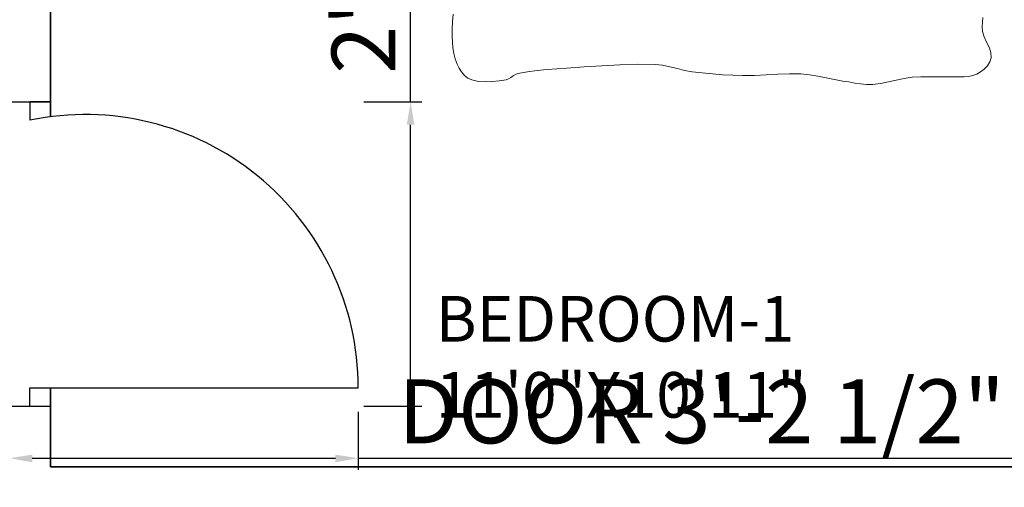
# Model space of a CAD drawing. Units: inches. Extents: x 1484 to 2008, y 1843 to 2590.
# Tile 11 of 21: x 1756 to 1864, y 2075 to 2126. Entities that reach past the tile are written whole.
import ezdxf

# ---------------------------------------------------------------- set-up
doc = ezdxf.new("R2010")
doc.units = ezdxf.units.IN
for name, color, linetype, lineweight in [('A-ANNO-DIMS', 2, 'Continuous', 18), ('A-AREA-IDEN', 7, 'Continuous', 18), ('A-DOOR', 4, 'Continuous', 25), ('A-FURN', 8, 'Continuous', 18), ('A-WALL', 7, 'Continuous', 35)]:
    doc.layers.add(name, color=color, linetype=linetype, lineweight=lineweight)
doc.styles.get("Standard").update_dxf_attribs({"font": 'arial.ttf'})
doc.dimstyles.new('ISO-25', dxfattribs={"dimtxt": 7, "dimasz": 2.5, "dimexe": 1.25, "dimexo": 0.625, "dimtad": 1, "dimdec": 0, "dimlunit": 3, "dimtxsty": 'Standard', "dimcen": 2.5, "dimadec": 0, "dimazin": 0, "dimtfac": 1, "dimtdec": 0, "dimtmove": 0, "dimatfit": 3, "dimfxl": 1, "dimarcsym": 0})

# ---------------------------------------------------------------- blocks, each defined once
blk = doc.blocks.new('BED-DOUBLE')
for p, q in [((0.44, 7.72), (0.38, 6.9)), ((0.38, 6.9), (0.33, 6.08)), ((58.47, 6.32), (58.48, 6.84)), ((58.48, 6.84), (58.53, 7.36)), ((0.33, 6.08), (0.34, 5.26)), ((58.51, 5.8), (58.47, 6.32)), ((58.67, 5.21), (58.51, 5.8)), ((0.34, 5.26), (0.37, 4.64)), ((0.37, 4.64), (0.43, 4.02)), ((58.94, 4.64), (58.67, 5.21)), ((59.21, 4.08), (58.94, 4.64)), ((0.43, 4.02), (0.52, 3.41)), ((0.52, 3.41), (0.66, 2.81)), ((59.41, 3.51), (59.21, 4.08)), ((59.44, 2.92), (59.41, 3.51)), ((0.66, 2.81), (0.87, 2.24)), ((0.87, 2.24), (1.09, 1.8)), ((16.76, 2.06), (18.71, 2.17)), ((18.71, 2.17), (20.65, 2.22)), ((20.65, 2.22), (22.59, 2.2)), ((22.59, 2.2), (23.41, 2.12)), ((59.04, 2.06), (59.3, 2.47)), ((59.3, 2.47), (59.44, 2.92)), ((1.09, 1.8), (1.37, 1.38)), ((1.37, 1.38), (1.69, 1)), ((7.03, 0.95), (7.28, 1.11)), ((7.28, 1.11), (7.55, 1.21)), ((7.55, 1.21), (8.61, 1.39)), ((8.61, 1.39), (9.67, 1.53)), ((9.67, 1.53), (10.74, 1.64)), ((10.74, 1.64), (11.81, 1.73)), ((11.81, 1.73), (12.88, 1.8)), ((12.88, 1.8), (14.82, 1.94)), ((14.82, 1.94), (16.76, 2.06)), ((23.41, 2.12), (24.22, 1.95)), ((24.22, 1.95), (25.03, 1.75)), ((25.03, 1.75), (25.83, 1.54)), ((25.83, 1.54), (26.65, 1.4)), ((26.65, 1.4), (27.76, 1.27)), ((27.76, 1.27), (28.88, 1.16)), ((28.88, 1.16), (29.99, 1.07)), ((34.77, 1.05), (36.04, 1.13)), ((36.04, 1.13), (37.32, 1.18)), ((37.32, 1.18), (38.59, 1.16)), ((38.59, 1.16), (39.51, 1.07)), ((57.43, 0.97), (57.87, 1.14)), ((57.87, 1.14), (58.29, 1.39)), ((58.29, 1.39), (58.69, 1.7)), ((58.69, 1.7), (59.04, 2.06)), ((1.69, 1), (2.07, 0.7)), ((2.07, 0.7), (2.5, 0.5)), ((2.5, 0.5), (3.23, 0.34)), ((3.23, 0.34), (3.98, 0.29)), ((3.98, 0.29), (4.74, 0.33)), ((4.74, 0.33), (5.5, 0.41)), ((5.5, 0.41), (6.25, 0.52)), ((6.25, 0.52), (6.53, 0.61)), ((6.53, 0.61), (6.78, 0.77)), ((6.78, 0.77), (7.03, 0.95)), ((29.99, 1.07), (31.11, 1.01)), ((31.11, 1.01), (32.23, 0.97)), ((32.23, 0.97), (33.5, 0.99)), ((33.5, 0.99), (34.77, 1.05)), ((39.51, 1.07), (40.43, 0.92)), ((40.43, 0.92), (41.35, 0.73)), ((41.35, 0.73), (42.27, 0.54)), ((42.27, 0.54), (43.19, 0.38)), ((43.19, 0.38), (43.83, 0.28)), ((43.83, 0.28), (44.48, 0.16)), ((44.48, 0.16), (45.13, 0.06)), ((45.13, 0.06), (45.77, 0)), ((45.77, 0), (46.42, 0)), ((46.42, 0), (47.3, 0.1)), ((47.3, 0.1), (48.17, 0.28)), ((48.17, 0.28), (49.04, 0.48)), ((49.04, 0.48), (49.91, 0.67)), ((49.91, 0.67), (50.79, 0.8)), ((50.79, 0.8), (51.74, 0.85)), ((51.74, 0.85), (52.68, 0.86)), ((52.68, 0.86), (53.63, 0.84)), ((53.63, 0.84), (54.58, 0.83)), ((54.58, 0.83), (55.53, 0.85)), ((55.53, 0.85), (56.01, 0.86)), ((56.01, 0.86), (56.49, 0.86)), ((56.49, 0.86), (56.97, 0.89)), ((56.97, 0.89), (57.43, 0.97))]:
    blk.add_line(p, q)
blk = doc.blocks.new('DOOR-SWING-36IN')
for p, q in [((-2.25, 31.33), (2.25, 31.33)), ((0, 31.33), (0, 29.33)), ((0, -2), (0, 0)), ((0, 0), (36, 0)), ((-2.25, -2), (2.25, -2))]:
    blk.add_line(p, q)
blk.add_arc((6.05, 0), 29.95, 0, 101.6643)
blk = doc.blocks.new('*D11')
at = {"layer": 'A-ANNO-DIMS', "color": 0, "lineweight": -2, "transparency": 16777216}
for p, q in [((1754.42, 2083.34), (1754.42, 2076.98)), ((1792.67, 2083.34), (1792.67, 2076.98)), ((1756.92, 2078.23), (1790.17, 2078.23)), ((1792.67, 2078.23), (1887.1, 2078.23))]:
    blk.add_line(p, q, dxfattribs=at)
at = {"layer": 'A-ANNO-DIMS', "color": 0, "transparency": 16777216}
for points in [[(1756.92, 2078.64), (1756.92, 2077.81), (1754.42, 2078.23)], [(1790.17, 2078.64), (1790.17, 2077.81), (1792.67, 2078.23)]]:
    blk.add_solid(points, dxfattribs=at)
at = {"layer": 'Defpoints', "color": 0, "transparency": 16777216}
for p in [(1754.42, 2083.96), (1792.67, 2083.96), (1792.67, 2078.23)]:
    blk.add_point(p, dxfattribs=at)
at = {"layer": 'A-ANNO-DIMS', "color": 0, "transparency": 16777216, "insert": (1841.14, 2082.47), "char_height": 7, "attachment_point": 5}
blk.add_mtext('DOOR 3\'-2 1/2" TYP.', dxfattribs=at)
blk = doc.blocks.new('*D12')
at = {"layer": 'A-ANNO-DIMS', "color": 0, "lineweight": -2, "transparency": 16777216}
for p, q in [((1798.41, 2117.29), (1798.41, 2180.14)), ((1793.29, 2117.29), (1799.66, 2117.29)), ((1798.41, 2086.46), (1798.41, 2114.79)), ((1793.29, 2083.96), (1799.66, 2083.96))]:
    blk.add_line(p, q, dxfattribs=at)
at = {"layer": 'A-ANNO-DIMS', "color": 0, "transparency": 16777216}
for points in [[(1797.99, 2114.79), (1798.82, 2114.79), (1798.41, 2117.29)], [(1797.99, 2086.46), (1798.82, 2086.46), (1798.41, 2083.96)]]:
    blk.add_solid(points, dxfattribs=at)
at = {"layer": 'Defpoints', "color": 0, "transparency": 16777216}
for p in [(1792.67, 2117.29), (1798.41, 2117.29), (1792.67, 2083.96)]:
    blk.add_point(p, dxfattribs=at)
at = {"layer": 'A-ANNO-DIMS', "color": 0, "transparency": 16777216, "insert": (1794.16, 2149.96), "char_height": 7, "attachment_point": 5, "rotation": 90}
blk.add_mtext('2\'-9 1/2" TYP.', dxfattribs=at)

msp = doc.modelspace()

# ---------------------------------------------------------------- linework, layer by layer
at = {"layer": 'A-DOOR'}
msp.add_line((1758.92, 2117.29), (1756.67, 2117.29), dxfattribs=at)
at = {"layer": 'A-WALL'}
for p, q in [((1758.92, 2208.3), (1758.92, 2115.67)), ((1758.92, 2085.96), (1758.92, 2077.3)), ((1758.92, 2077.3), (1890.92, 2077.3))]:
    msp.add_line(p, q, dxfattribs=at)

# ---------------------------------------------------------------- block references
at = {"layer": 'A-DOOR'}
msp.add_blockref('DOOR-SWING-36IN', (1756.67, 2085.96), dxfattribs=at)
at = {"layer": 'A-FURN'}
msp.add_blockref('BED-DOUBLE', (1802.63, 2119.2), dxfattribs=at)

# ---------------------------------------------------------------- texts
at = {"layer": 'A-AREA-IDEN', "insert": (1801.17, 2096.02), "char_height": 5, "attachment_point": 1}
msp.add_mtext_dynamic_manual_height_columns('BEDROOM-1\\P11\'0"X10\'11"', width=115.7673, gutter_width=12.5, heights=[0], dxfattribs=at)

# ---------------------------------------------------------------- dimensions: what is measured, and where the dimension line sits
at = {"layer": 'A-ANNO-DIMS'}
dim = msp.add_linear_dim(base=(1798.41, 2117.29), p1=(1792.67, 2083.96), p2=(1792.67, 2117.29), angle=90, text='<> TYP.', dimstyle='ISO-25', override={"dimdec": 1, "dimlfac": 1, "dimrnd": 0, "dimzin": 1, "dimdsep": 46, "dimlunit": 4, "dimfrac": 2}, dxfattribs=at)
dim.commit()
dim.dimension.update_dxf_attribs({"geometry": '*D12', "text_midpoint": (1794.16, 2149.96)})
dim = msp.add_linear_dim(base=(1792.66964371, 2078.22557639), p1=(1754.41964371, 2083.96307639), p2=(1792.66964371, 2083.96307639), text='DOOR <> TYP.', dimstyle='ISO-25', override={"dimdec": 1, "dimlfac": 1, "dimrnd": 0, "dimzin": 1, "dimdsep": 46, "dimlunit": 4, "dimfrac": 2}, dxfattribs=at)
dim.commit()
dim.dimension.update_dxf_attribs({"geometry": '*D11', "text_midpoint": (1841.13707208, 2082.47472373)})

doc.saveas('drawing.dxf')
